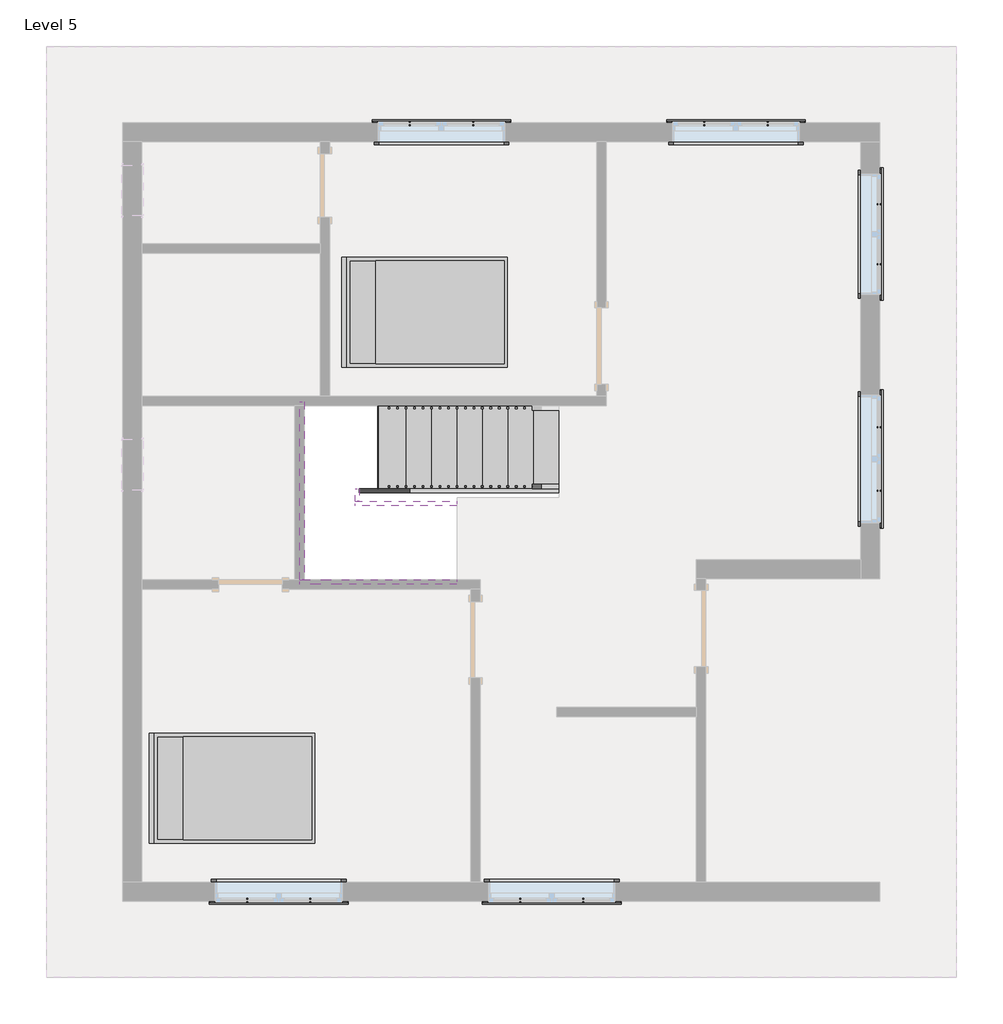
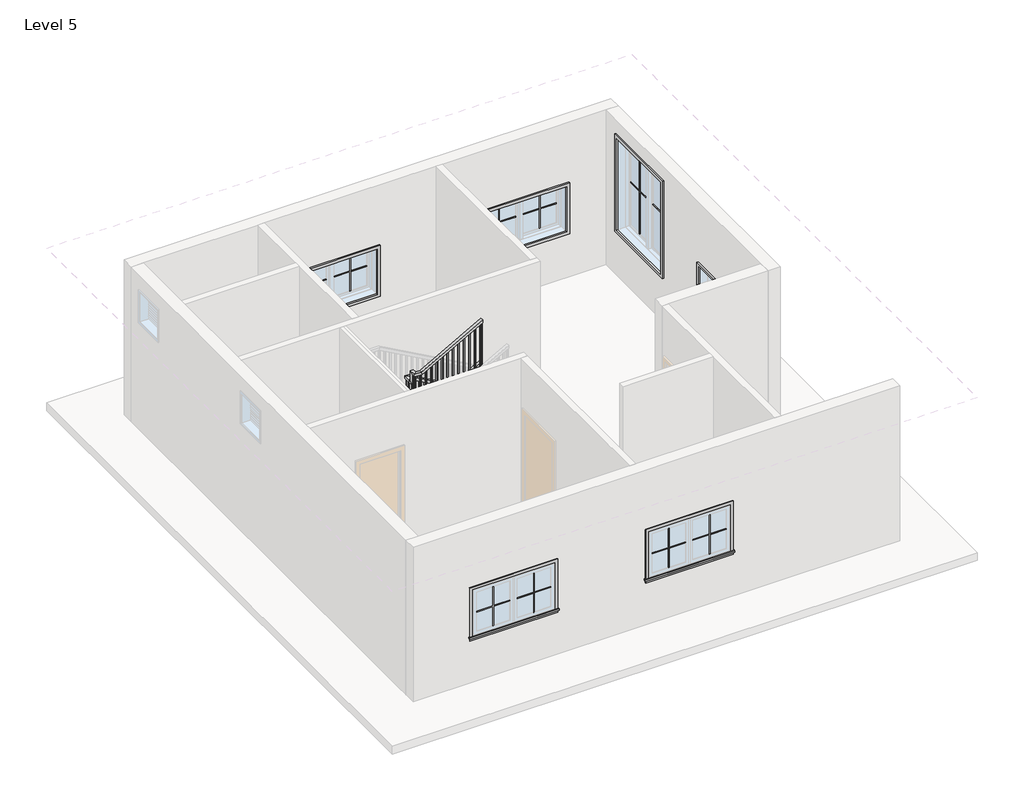
# One storey, part 2 of 2: 24 proxies, 6 members, 2 furniture elements, 1 railing, 1 stair flight.
"""IFC4 building model written with IfcOpenShell, lengths in millimetres."""

from ifc_helpers import new_model, si_unit, frame, origin, place, context, project, spatial, polyline, outline, extrude, faceted_brep, transform, mapped, element, save
from components import muntin_pattern_2x2_muntin_pattern_2x2_9352d081, muntin_pattern_2x2_muntin_pattern_2x2_5c2cbe28, muntin_pattern_2x2_muntin_pattern_2x2_bff912c5, muntin_pattern_2x2_muntin_pattern_2x2_c2194282, trim_window_exterior_flat_with_sill_979bde60, trim_window_exterior_flat_with_sill_e04b3088, trim_window_interior_flat_picture_frame_7883d11b, trim_window_interior_flat_picture_frame_2a7685fe, bed_17739_bed_17739_15c61121, stair_flight_2d4ab5d3

model = new_model("IFC4")

# Units and contexts
model_context = context("Model", 3, world=origin())
ifc_project = project(units=[si_unit("LENGTHUNIT", "METRE", prefix="MILLI")], contexts=[model_context])

# Site, building, storey
site = spatial("IfcSite", under=ifc_project)
building = spatial("IfcBuilding", under=site)
storey = spatial("IfcBuildingStorey", under=building, Name="Level 5", Elevation=12649.2)

# Proxies
placement = place(None, origin())
muntin_pattern_2x2_muntin_pattern_2x2_shape = muntin_pattern_2x2_muntin_pattern_2x2_9352d081(model_context)
element("IfcBuildingElementProxy", 1, Name="Muntin Pattern_2x2 : Muntin Pattern_2x2", ObjectType="Muntin Pattern_2x2 : Muntin Pattern_2x2", at=placement, inside=storey, context=model_context, shape_type="MappedRepresentation", body=[
    mapped(muntin_pattern_2x2_muntin_pattern_2x2_shape, transform((-3542.9505704, -5264.0292021, 13633.45), x_axis=(-1.0, 0.0, 0.0), y_axis=(0.0, -1.0, 0.0), z_axis=(0.0, 0.0, 1.0))),
])
element("IfcBuildingElementProxy", 2, Name="Muntin Pattern_2x2 : Muntin Pattern_2x2", ObjectType="Muntin Pattern_2x2 : Muntin Pattern_2x2", at=placement, inside=storey, context=model_context, shape_type="MappedRepresentation", body=[
    mapped(muntin_pattern_2x2_muntin_pattern_2x2_shape, transform((-272.7005704, -5264.0292021, 13633.45), x_axis=(-1.0, 0.0, 0.0), y_axis=(0.0, -1.0, 0.0), z_axis=(0.0, 0.0, 1.0))),
])
element("IfcBuildingElementProxy", 3, Name="Muntin Pattern_2x2 : Muntin Pattern_2x2", ObjectType="Muntin Pattern_2x2 : Muntin Pattern_2x2", at=placement, inside=storey, context=model_context, shape_type="MappedRepresentation", body=[
    mapped(muntin_pattern_2x2_muntin_pattern_2x2_shape, transform((3269.0119296, 401.7582979, 13633.45), x_axis=(0.0, -1.0, 0.0), y_axis=(1.0, 0.0, 0.0), z_axis=(0.0, 0.0, 1.0))),
])
element("IfcBuildingElementProxy", 4, Name="Muntin Pattern_2x2 : Muntin Pattern_2x2", ObjectType="Muntin Pattern_2x2 : Muntin Pattern_2x2", at=placement, inside=storey, context=model_context, shape_type="MappedRepresentation", body=[
    mapped(muntin_pattern_2x2_muntin_pattern_2x2_shape, transform((1175.0994296, 4038.7207979, 13633.45), x_axis=(1.0, 0.0, 0.0), y_axis=(0.0, 1.0, 0.0), z_axis=(0.0, 0.0, 1.0))),
])
element("IfcBuildingElementProxy", 5, Name="Muntin Pattern_2x2 : Muntin Pattern_2x2", ObjectType="Muntin Pattern_2x2 : Muntin Pattern_2x2", at=placement, inside=storey, context=model_context, shape_type="MappedRepresentation", body=[
    mapped(muntin_pattern_2x2_muntin_pattern_2x2_shape, transform((-2352.3255704, 4038.7207979, 13633.45), x_axis=(1.0, 0.0, 0.0), y_axis=(0.0, 1.0, 0.0), z_axis=(0.0, 0.0, 1.0))),
])
muntin_pattern_2x2_muntin_pattern_2x2_2_shape = muntin_pattern_2x2_muntin_pattern_2x2_5c2cbe28(model_context)
element("IfcBuildingElementProxy", 6, Name="Muntin Pattern_2x2 : Muntin Pattern_2x2", ObjectType="Muntin Pattern_2x2 : Muntin Pattern_2x2", at=placement, inside=storey, context=model_context, shape_type="MappedRepresentation", body=[
    mapped(muntin_pattern_2x2_muntin_pattern_2x2_2_shape, transform((-4301.7755704, -5264.0292021, 13633.45), x_axis=(1.0, 0.0, 0.0), y_axis=(0.0, 1.0, 0.0), z_axis=(0.0, 0.0, 1.0))),
])
element("IfcBuildingElementProxy", 7, Name="Muntin Pattern_2x2 : Muntin Pattern_2x2", ObjectType="Muntin Pattern_2x2 : Muntin Pattern_2x2", at=placement, inside=storey, context=model_context, shape_type="MappedRepresentation", body=[
    mapped(muntin_pattern_2x2_muntin_pattern_2x2_2_shape, transform((-1031.5255704, -5264.0292021, 13633.45), x_axis=(1.0, 0.0, 0.0), y_axis=(0.0, 1.0, 0.0), z_axis=(0.0, 0.0, 1.0))),
])
element("IfcBuildingElementProxy", 8, Name="Muntin Pattern_2x2 : Muntin Pattern_2x2", ObjectType="Muntin Pattern_2x2 : Muntin Pattern_2x2", at=placement, inside=storey, context=model_context, shape_type="MappedRepresentation", body=[
    mapped(muntin_pattern_2x2_muntin_pattern_2x2_2_shape, transform((3269.0119296, -357.0667021, 13633.45), x_axis=(0.0, 1.0, 0.0), y_axis=(-1.0, 0.0, 0.0), z_axis=(0.0, 0.0, 1.0))),
])
element("IfcBuildingElementProxy", 9, Name="Muntin Pattern_2x2 : Muntin Pattern_2x2", ObjectType="Muntin Pattern_2x2 : Muntin Pattern_2x2", at=placement, inside=storey, context=model_context, shape_type="MappedRepresentation", body=[
    mapped(muntin_pattern_2x2_muntin_pattern_2x2_2_shape, transform((1933.9244296, 4038.7207979, 13633.45), x_axis=(-1.0, 0.0, 0.0), y_axis=(0.0, -1.0, 0.0), z_axis=(0.0, 0.0, 1.0))),
])
element("IfcBuildingElementProxy", 10, Name="Muntin Pattern_2x2 : Muntin Pattern_2x2", ObjectType="Muntin Pattern_2x2 : Muntin Pattern_2x2", at=placement, inside=storey, context=model_context, shape_type="MappedRepresentation", body=[
    mapped(muntin_pattern_2x2_muntin_pattern_2x2_2_shape, transform((-1593.5005704, 4038.7207979, 13633.45), x_axis=(-1.0, 0.0, 0.0), y_axis=(0.0, -1.0, 0.0), z_axis=(0.0, 0.0, 1.0))),
])
muntin_pattern_2x2_muntin_pattern_2x2_3_shape = muntin_pattern_2x2_muntin_pattern_2x2_bff912c5(model_context)
element("IfcBuildingElementProxy", 11, Name="Muntin Pattern_2x2 : Muntin Pattern_2x2", ObjectType="Muntin Pattern_2x2 : Muntin Pattern_2x2", at=placement, inside=storey, context=model_context, shape_type="MappedRepresentation", body=[
    mapped(muntin_pattern_2x2_muntin_pattern_2x2_3_shape, transform((3269.0119296, 3075.1082979, 13633.45), x_axis=(0.0, -1.0, 0.0), y_axis=(1.0, 0.0, 0.0), z_axis=(0.0, 0.0, 1.0))),
])
muntin_pattern_2x2_muntin_pattern_2x2_4_shape = muntin_pattern_2x2_muntin_pattern_2x2_c2194282(model_context)
element("IfcBuildingElementProxy", 12, Name="Muntin Pattern_2x2 : Muntin Pattern_2x2", ObjectType="Muntin Pattern_2x2 : Muntin Pattern_2x2", at=placement, inside=storey, context=model_context, shape_type="MappedRepresentation", body=[
    mapped(muntin_pattern_2x2_muntin_pattern_2x2_4_shape, transform((3269.0119296, 2354.3832979, 13633.45), x_axis=(0.0, 1.0, 0.0), y_axis=(-1.0, 0.0, 0.0), z_axis=(0.0, 0.0, 1.0))),
])
trim_window_exterior_flat_with_sill_shape = trim_window_exterior_flat_with_sill_979bde60(model_context)
element("IfcBuildingElementProxy", 13, Name="Trim-Window-Exterior-Flat : with Sill", ObjectType="Trim-Window-Exterior-Flat : with Sill", at=placement, inside=storey, context=model_context, shape_type="MappedRepresentation", body=[
    mapped(trim_window_exterior_flat_with_sill_shape, transform((-3922.3630704, -5273.5542021, 14478.0), x_axis=(1.0, 0.0, 0.0), y_axis=(0.0, 0.0, 1.0), z_axis=(0.0, -1.0, 0.0))),
])
element("IfcBuildingElementProxy", 14, Name="Trim-Window-Exterior-Flat : with Sill", ObjectType="Trim-Window-Exterior-Flat : with Sill", at=placement, inside=storey, context=model_context, shape_type="MappedRepresentation", body=[
    mapped(trim_window_exterior_flat_with_sill_shape, transform((-652.1130704, -5273.5542021, 14478.0), x_axis=(1.0, 0.0, 0.0), y_axis=(0.0, 0.0, 1.0), z_axis=(0.0, -1.0, 0.0))),
])
element("IfcBuildingElementProxy", 15, Name="Trim-Window-Exterior-Flat : with Sill", ObjectType="Trim-Window-Exterior-Flat : with Sill", at=placement, inside=storey, context=model_context, shape_type="MappedRepresentation", body=[
    mapped(trim_window_exterior_flat_with_sill_shape, transform((3278.5369296, 22.3457979, 14478.0), x_axis=(0.0, 1.0, 0.0), y_axis=(0.0, 0.0, 1.0), z_axis=(1.0, 0.0, 0.0))),
])
element("IfcBuildingElementProxy", 16, Name="Trim-Window-Exterior-Flat : with Sill", ObjectType="Trim-Window-Exterior-Flat : with Sill", at=placement, inside=storey, context=model_context, shape_type="MappedRepresentation", body=[
    mapped(trim_window_exterior_flat_with_sill_shape, transform((1554.5119296, 4048.2457979, 14478.0), x_axis=(-1.0, 0.0, 0.0), y_axis=(0.0, 0.0, 1.0), z_axis=(0.0, 1.0, 0.0))),
])
element("IfcBuildingElementProxy", 17, Name="Trim-Window-Exterior-Flat : with Sill", ObjectType="Trim-Window-Exterior-Flat : with Sill", at=placement, inside=storey, context=model_context, shape_type="MappedRepresentation", body=[
    mapped(trim_window_exterior_flat_with_sill_shape, transform((-1972.9130704, 4048.2457979, 14478.0), x_axis=(-1.0, 0.0, 0.0), y_axis=(0.0, 0.0, 1.0), z_axis=(0.0, 1.0, 0.0))),
])
trim_window_exterior_flat_with_sill_2_shape = trim_window_exterior_flat_with_sill_e04b3088(model_context)
element("IfcBuildingElementProxy", 18, Name="Trim-Window-Exterior-Flat : with Sill", ObjectType="Trim-Window-Exterior-Flat : with Sill", at=placement, inside=storey, context=model_context, shape_type="MappedRepresentation", body=[
    mapped(trim_window_exterior_flat_with_sill_2_shape, transform((3278.5369296, 2714.7457979, 15392.4), x_axis=(0.0, 1.0, 0.0), y_axis=(0.0, 0.0, 1.0), z_axis=(1.0, 0.0, 0.0))),
])
trim_window_interior_flat_picture_frame_shape = trim_window_interior_flat_picture_frame_7883d11b(model_context)
element("IfcBuildingElementProxy", 19, Name="Trim-Window-Interior-Flat : Picture Frame", ObjectType="Trim-Window-Interior-Flat : Picture Frame", at=placement, inside=storey, context=model_context, shape_type="MappedRepresentation", body=[
    mapped(trim_window_interior_flat_picture_frame_shape, transform((-3922.3630704, -5044.9542021, 14478.0), x_axis=(-1.0, 0.0, 0.0), y_axis=(0.0, 0.0, 1.0), z_axis=(0.0, 1.0, 0.0))),
])
element("IfcBuildingElementProxy", 20, Name="Trim-Window-Interior-Flat : Picture Frame", ObjectType="Trim-Window-Interior-Flat : Picture Frame", at=placement, inside=storey, context=model_context, shape_type="MappedRepresentation", body=[
    mapped(trim_window_interior_flat_picture_frame_shape, transform((-652.1130704, -5044.9542021, 14478.0), x_axis=(-1.0, 0.0, 0.0), y_axis=(0.0, 0.0, 1.0), z_axis=(0.0, 1.0, 0.0))),
])
element("IfcBuildingElementProxy", 21, Name="Trim-Window-Interior-Flat : Picture Frame", ObjectType="Trim-Window-Interior-Flat : Picture Frame", at=placement, inside=storey, context=model_context, shape_type="MappedRepresentation", body=[
    mapped(trim_window_interior_flat_picture_frame_shape, transform((3049.9369296, 22.3457979, 14478.0), x_axis=(0.0, -1.0, 0.0), y_axis=(0.0, 0.0, 1.0), z_axis=(-1.0, 0.0, 0.0))),
])
element("IfcBuildingElementProxy", 22, Name="Trim-Window-Interior-Flat : Picture Frame", ObjectType="Trim-Window-Interior-Flat : Picture Frame", at=placement, inside=storey, context=model_context, shape_type="MappedRepresentation", body=[
    mapped(trim_window_interior_flat_picture_frame_shape, transform((1554.5119296, 3819.6457979, 14478.0), x_axis=(1.0, 0.0, 0.0), y_axis=(0.0, 0.0, 1.0), z_axis=(0.0, -1.0, 0.0))),
])
element("IfcBuildingElementProxy", 23, Name="Trim-Window-Interior-Flat : Picture Frame", ObjectType="Trim-Window-Interior-Flat : Picture Frame", at=placement, inside=storey, context=model_context, shape_type="MappedRepresentation", body=[
    mapped(trim_window_interior_flat_picture_frame_shape, transform((-1972.9130704, 3819.6457979, 14478.0), x_axis=(1.0, 0.0, 0.0), y_axis=(0.0, 0.0, 1.0), z_axis=(0.0, -1.0, 0.0))),
])
trim_window_interior_flat_picture_frame_2_shape = trim_window_interior_flat_picture_frame_2a7685fe(model_context)
element("IfcBuildingElementProxy", 24, Name="Trim-Window-Interior-Flat : Picture Frame", ObjectType="Trim-Window-Interior-Flat : Picture Frame", at=placement, inside=storey, context=model_context, shape_type="MappedRepresentation", body=[
    mapped(trim_window_interior_flat_picture_frame_2_shape, transform((3049.9369296, 2714.7457979, 15392.4), x_axis=(0.0, -1.0, 0.0), y_axis=(0.0, 0.0, 1.0), z_axis=(-1.0, 0.0, 0.0))),
])

# Furniture
bed_17739_bed_17739_shape = bed_17739_bed_17739_15c61121(model_context)
element("IfcFurniture", 25, ObjectType="Bed_17739 : Bed_17739", at=placement, inside=storey, context=model_context, shape_type="MappedRepresentation", body=[
    mapped(bed_17739_bed_17739_shape, transform((-4455.7630704, -3920.5467683, 12649.2), x_axis=(0.0, 1.0, 0.0), y_axis=(-1.0, 0.0, 0.0), z_axis=(0.0, 0.0, 1.0))),
])
element("IfcFurniture", 26, ObjectType="Bed_17739 : Bed_17739", at=placement, inside=storey, context=model_context, shape_type="MappedRepresentation", body=[
    mapped(bed_17739_bed_17739_shape, transform((-2150.7130704, 1781.2957979, 12649.2), x_axis=(0.0, 1.0, 0.0), y_axis=(-1.0, 0.0, 0.0), z_axis=(0.0, 0.0, 1.0))),
])

# Members
element("IfcMember", 27, ObjectType="Stringer - 2\" Width", at=placement, inside=storey, context=model_context, shape_type="SweptSolid", body=[
    extrude(outline(polyline([(12649.2, -569.5630704), (12856.7983948, -569.5630704), (14183.2428392, -2957.1630704), (13834.5641651, -2957.1630704), (12649.2, -823.5075732), (12649.2, -569.5630704)])), frame((0.0, -384.0542021, 0.0), z_axis=(0.0, 1.0, 0.0), x_axis=(0.0, 0.0, 1.0)), (0.0, 0.0, 1.0), 50.8),
])
element("IfcMember", 28, ObjectType="Stringer - 2\" Width", at=placement, inside=storey, context=model_context, shape_type="SweptSolid", body=[
    extrude(outline(polyline([(-3007.9630704, -333.2542021), (-2957.1630704, -333.2542021), (-2957.1630704, -485.6542021), (-3007.9630704, -485.6542021), (-3007.9630704, -333.2542021)])), frame((0.0, 0.0, 13944.6), z_axis=(0.0, 0.0, 1.0), x_axis=(1.0, 0.0, 0.0)), (0.0, 0.0, 1.0), 304.8),
])
element("IfcMember", 29, ObjectType="Stringer - 2\" Width", at=placement, inside=storey, context=model_context, shape_type="SweptSolid", body=[
    extrude(outline(polyline([(14380.7983948, -3007.9630704), (14032.1197207, -3007.9630704), (14709.453054, -1788.7630704), (15058.1317281, -1788.7630704), (14380.7983948, -3007.9630704)])), frame((0.0, -536.4542021, 0.0), z_axis=(0.0, 1.0, 0.0), x_axis=(0.0, 0.0, 1.0)), (0.0, 0.0, 1.0), 50.8),
])
element("IfcMember", 30, ObjectType="Stringer - 2\" Width", at=placement, inside=storey, context=model_context, shape_type="SweptSolid", body=[
    extrude(outline(polyline([(12649.2, -569.5630704), (12856.7983948, -569.5630704), (14249.4, -3076.2459598), (14249.4, -3617.5630704), (14201.453054, -3617.5630704), (12649.2, -823.5075732), (12649.2, -569.5630704)])), frame((0.0, 657.3457979, 0.0), z_axis=(0.0, 1.0, 0.0), x_axis=(0.0, 0.0, 1.0)), (0.0, 0.0, 1.0), 50.8),
])
element("IfcMember", 31, ObjectType="Stringer - 2\" Width", at=placement, inside=storey, context=model_context, shape_type="SweptSolid", body=[
    extrude(outline(polyline([(-3668.3630704, 708.1457979), (-3617.5630704, 708.1457979), (-3617.5630704, -1425.4542021), (-3668.3630704, -1425.4542021), (-3668.3630704, 708.1457979)])), frame((0.0, 0.0, 13944.6), z_axis=(0.0, 0.0, 1.0), x_axis=(1.0, 0.0, 0.0)), (0.0, 0.0, 1.0), 304.8),
])
element("IfcMember", 32, ObjectType="Stringer - 2\" Width", at=placement, inside=storey, context=model_context, shape_type="SweptSolid", body=[
    extrude(outline(polyline([(14013.9095059, -3668.3630704), (13944.6, -3668.3630704), (13944.6, -3165.4985677), (14709.453054, -1788.7630704), (15058.1317281, -1788.7630704), (14013.9095059, -3668.3630704)])), frame((0.0, -1476.2542021, 0.0), z_axis=(0.0, 1.0, 0.0), x_axis=(0.0, 0.0, 1.0)), (0.0, 0.0, 1.0), 50.8),
])

# Railing
element("IfcRailing", 33, ObjectType="Handrail - Rectangular", at=placement, inside=storey, context=model_context, shape_type="SolidModel", body=[
    faceted_brep([(-569.5630704, -333.2542021, 13732.9333333), (-569.5630704, -333.2542021, 13674.820221), (-569.5630704, -282.4542021, 13674.820221), (-569.5630704, -282.4542021, 13732.9333333), (-2931.7630704, -333.2542021, 15045.2666667), (-2982.5630704, -333.2542021, 15015.3757765), (-2982.5630704, -282.4542021, 15015.3757765), (-2931.7630704, -282.4542021, 15045.2666667), (-2931.7630704, -333.2542021, 15087.6), (-2982.5630704, -333.2542021, 15036.8), (-2982.5630704, -282.4542021, 15036.8), (-2931.7630704, -282.4542021, 15087.6), (-3007.9630704, -333.2542021, 15087.6), (-3007.9630704, -333.2542021, 15036.8), (-3058.7630704, -282.4542021, 15036.8), (-3058.7630704, -282.4542021, 15087.6), (-3007.9630704, -409.4542021, 15087.6), (-3007.9630704, -409.4542021, 15036.8), (-3058.7630704, -409.4542021, 15036.8), (-3058.7630704, -409.4542021, 15087.6), (-3007.9630704, -460.2542021, 15087.6), (-3007.9630704, -511.0542021, 15036.8), (-3058.7630704, -511.0542021, 15036.8), (-3058.7630704, -460.2542021, 15087.6), (-3007.9630704, -460.2542021, 15299.2666667), (-3007.9630704, -511.0542021, 15248.4666667), (-3058.7630704, -511.0542021, 15248.4666667), (-3058.7630704, -460.2542021, 15299.2666667), (-3007.9630704, -536.4542021, 15299.2666667), (-3007.9630704, -536.4542021, 15248.4666667), (-3058.7630704, -587.2542021, 15248.4666667), (-3058.7630704, -587.2542021, 15299.2666667), (-2931.7630704, -536.4542021, 15299.2666667), (-2918.5994682, -536.4542021, 15248.4666667), (-2918.5994682, -587.2542021, 15248.4666667), (-2931.7630704, -587.2542021, 15299.2666667), (-1788.7630704, -536.4542021, 15934.2666667), (-1788.7630704, -587.2542021, 15934.2666667), (-1788.7630704, -587.2542021, 15876.1535543), (-1788.7630704, -536.4542021, 15876.1535543)], [[[0, 1, 2, 3]], [[1, 0, 4, 5]], [[2, 1, 5, 6]], [[3, 2, 6, 7]], [[0, 3, 7, 4]], [[5, 4, 8, 9]], [[6, 5, 9, 10]], [[7, 6, 10, 11]], [[4, 7, 11, 8]], [[9, 8, 12, 13]], [[10, 9, 13, 14]], [[11, 10, 14, 15]], [[8, 11, 15, 12]], [[13, 12, 16, 17]], [[14, 13, 17, 18]], [[15, 14, 18, 19]], [[12, 15, 19, 16]], [[17, 16, 20, 21]], [[18, 17, 21, 22]], [[19, 18, 22, 23]], [[16, 19, 23, 20]], [[21, 20, 24, 25]], [[22, 21, 25, 26]], [[23, 22, 26, 27]], [[20, 23, 27, 24]], [[25, 24, 28, 29]], [[26, 25, 29, 30]], [[27, 26, 30, 31]], [[24, 27, 31, 28]], [[29, 28, 32, 33]], [[30, 29, 33, 34]], [[31, 30, 34, 35]], [[28, 31, 35, 32]], [[36, 37, 38, 39]], [[33, 32, 36, 39]], [[34, 33, 39, 38]], [[35, 34, 38, 37]], [[32, 35, 37, 36]]]),
    extrude(outline(polyline([(15856.7507765, -1823.6880704), (14850.5333333, -1823.6880704), (14850.5333333, -1804.6380704), (15867.3341099, -1804.6380704), (15856.7507765, -1823.6880704)])), frame((0.0, -571.3792021, 0.0), z_axis=(0.0, 1.0, 0.0), x_axis=(0.0, 0.0, 1.0)), (0.0, 0.0, 1.0), 19.05),
    extrude(outline(polyline([(15800.3063321, -1925.2880704), (14850.5333333, -1925.2880704), (14850.5333333, -1906.2380704), (15810.8896654, -1906.2380704), (15800.3063321, -1925.2880704)])), frame((0.0, -571.3792021, 0.0), z_axis=(0.0, 1.0, 0.0), x_axis=(0.0, 0.0, 1.0)), (0.0, 0.0, 1.0), 19.05),
    extrude(outline(polyline([(15743.8618876, -2026.8880704), (14850.5333333, -2026.8880704), (14850.5333333, -2007.8380704), (15754.445221, -2007.8380704), (15743.8618876, -2026.8880704)])), frame((0.0, -571.3792021, 0.0), z_axis=(0.0, 1.0, 0.0), x_axis=(0.0, 0.0, 1.0)), (0.0, 0.0, 1.0), 19.05),
    extrude(outline(polyline([(15687.4174432, -2128.4880704), (14681.2, -2128.4880704), (14681.2, -2109.4380704), (15698.0007765, -2109.4380704), (15687.4174432, -2128.4880704)])), frame((0.0, -571.3792021, 0.0), z_axis=(0.0, 1.0, 0.0), x_axis=(0.0, 0.0, 1.0)), (0.0, 0.0, 1.0), 19.05),
    extrude(outline(polyline([(15630.9729988, -2230.0880704), (14681.2, -2230.0880704), (14681.2, -2211.0380704), (15641.5563321, -2211.0380704), (15630.9729988, -2230.0880704)])), frame((0.0, -571.3792021, 0.0), z_axis=(0.0, 1.0, 0.0), x_axis=(0.0, 0.0, 1.0)), (0.0, 0.0, 1.0), 19.05),
    extrude(outline(polyline([(15574.5285543, -2331.6880704), (14681.2, -2331.6880704), (14681.2, -2312.6380704), (15585.1118876, -2312.6380704), (15574.5285543, -2331.6880704)])), frame((0.0, -571.3792021, 0.0), z_axis=(0.0, 1.0, 0.0), x_axis=(0.0, 0.0, 1.0)), (0.0, 0.0, 1.0), 19.05),
    extrude(outline(polyline([(15518.0841099, -2433.2880704), (14511.8666667, -2433.2880704), (14511.8666667, -2414.2380704), (15528.6674432, -2414.2380704), (15518.0841099, -2433.2880704)])), frame((0.0, -571.3792021, 0.0), z_axis=(0.0, 1.0, 0.0), x_axis=(0.0, 0.0, 1.0)), (0.0, 0.0, 1.0), 19.05),
    extrude(outline(polyline([(15461.6396654, -2534.8880704), (14511.8666667, -2534.8880704), (14511.8666667, -2515.8380704), (15472.2229988, -2515.8380704), (15461.6396654, -2534.8880704)])), frame((0.0, -571.3792021, 0.0), z_axis=(0.0, 1.0, 0.0), x_axis=(0.0, 0.0, 1.0)), (0.0, 0.0, 1.0), 19.05),
    extrude(outline(polyline([(15405.195221, -2636.4880704), (14511.8666667, -2636.4880704), (14511.8666667, -2617.4380704), (15415.7785543, -2617.4380704), (15405.195221, -2636.4880704)])), frame((0.0, -571.3792021, 0.0), z_axis=(0.0, 1.0, 0.0), x_axis=(0.0, 0.0, 1.0)), (0.0, 0.0, 1.0), 19.05),
    extrude(outline(polyline([(15348.7507765, -2738.0880704), (14342.5333333, -2738.0880704), (14342.5333333, -2719.0380704), (15359.3341099, -2719.0380704), (15348.7507765, -2738.0880704)])), frame((0.0, -571.3792021, 0.0), z_axis=(0.0, 1.0, 0.0), x_axis=(0.0, 0.0, 1.0)), (0.0, 0.0, 1.0), 19.05),
    extrude(outline(polyline([(15292.3063321, -2839.6880704), (14342.5333333, -2839.6880704), (14342.5333333, -2820.6380704), (15302.8896654, -2820.6380704), (15292.3063321, -2839.6880704)])), frame((0.0, -571.3792021, 0.0), z_axis=(0.0, 1.0, 0.0), x_axis=(0.0, 0.0, 1.0)), (0.0, 0.0, 1.0), 19.05),
    extrude(outline(polyline([(15235.8618876, -2941.2880704), (14342.5333333, -2941.2880704), (14342.5333333, -2922.2380704), (15246.445221, -2922.2380704), (15235.8618876, -2941.2880704)])), frame((0.0, -571.3792021, 0.0), z_axis=(0.0, 1.0, 0.0), x_axis=(0.0, 0.0, 1.0)), (0.0, 0.0, 1.0), 19.05),
    extrude(outline(polyline([(-3023.8380704, -501.5292021), (-3023.8380704, -520.5792021), (-3042.8880704, -520.5792021), (-3042.8880704, -501.5292021), (-3023.8380704, -501.5292021)])), frame((0.0, 0.0, 14173.2), z_axis=(0.0, 0.0, 1.0), x_axis=(1.0, 0.0, 0.0)), (0.0, 0.0, 1.0), 1075.2666667),
    extrude(outline(polyline([(-3023.8380704, -399.9292021), (-3023.8380704, -418.9792021), (-3042.8880704, -418.9792021), (-3042.8880704, -399.9292021), (-3023.8380704, -399.9292021)])), frame((0.0, 0.0, 14173.2), z_axis=(0.0, 0.0, 1.0), x_axis=(1.0, 0.0, 0.0)), (0.0, 0.0, 1.0), 863.6),
    extrude(outline(polyline([(-2998.4380704, -317.3792021), (-3017.4880704, -317.3792021), (-3017.4880704, -298.3292021), (-2998.4380704, -298.3292021), (-2998.4380704, -317.3792021)])), frame((0.0, 0.0, 14173.2), z_axis=(0.0, 0.0, 1.0), x_axis=(1.0, 0.0, 0.0)), (0.0, 0.0, 1.0), 863.6),
    extrude(outline(polyline([(14978.3341099, -2915.8880704), (14003.8666667, -2915.8880704), (14003.8666667, -2896.8380704), (14967.7507765, -2896.8380704), (14978.3341099, -2915.8880704)])), frame((0.0, -317.3792021, 0.0), z_axis=(0.0, 1.0, 0.0), x_axis=(0.0, 0.0, 1.0)), (0.0, 0.0, 1.0), 19.05),
    extrude(outline(polyline([(14921.8896654, -2814.2880704), (14003.8666667, -2814.2880704), (14003.8666667, -2795.2380704), (14911.3063321, -2795.2380704), (14921.8896654, -2814.2880704)])), frame((0.0, -317.3792021, 0.0), z_axis=(0.0, 1.0, 0.0), x_axis=(0.0, 0.0, 1.0)), (0.0, 0.0, 1.0), 19.05),
    extrude(outline(polyline([(14865.445221, -2712.6880704), (14003.8666667, -2712.6880704), (14003.8666667, -2693.6380704), (14854.8618876, -2693.6380704), (14865.445221, -2712.6880704)])), frame((0.0, -317.3792021, 0.0), z_axis=(0.0, 1.0, 0.0), x_axis=(0.0, 0.0, 1.0)), (0.0, 0.0, 1.0), 19.05),
    extrude(outline(polyline([(14809.0007765, -2611.0880704), (13834.5333333, -2611.0880704), (13834.5333333, -2592.0380704), (14798.4174432, -2592.0380704), (14809.0007765, -2611.0880704)])), frame((0.0, -317.3792021, 0.0), z_axis=(0.0, 1.0, 0.0), x_axis=(0.0, 0.0, 1.0)), (0.0, 0.0, 1.0), 19.05),
    extrude(outline(polyline([(14752.5563321, -2509.4880704), (13834.5333333, -2509.4880704), (13834.5333333, -2490.4380704), (14741.9729988, -2490.4380704), (14752.5563321, -2509.4880704)])), frame((0.0, -317.3792021, 0.0), z_axis=(0.0, 1.0, 0.0), x_axis=(0.0, 0.0, 1.0)), (0.0, 0.0, 1.0), 19.05),
    extrude(outline(polyline([(14696.1118876, -2407.8880704), (13834.5333333, -2407.8880704), (13834.5333333, -2388.8380704), (14685.5285543, -2388.8380704), (14696.1118876, -2407.8880704)])), frame((0.0, -317.3792021, 0.0), z_axis=(0.0, 1.0, 0.0), x_axis=(0.0, 0.0, 1.0)), (0.0, 0.0, 1.0), 19.05),
    extrude(outline(polyline([(14639.6674432, -2306.2880704), (13665.2, -2306.2880704), (13665.2, -2287.2380704), (14629.0841099, -2287.2380704), (14639.6674432, -2306.2880704)])), frame((0.0, -317.3792021, 0.0), z_axis=(0.0, 1.0, 0.0), x_axis=(0.0, 0.0, 1.0)), (0.0, 0.0, 1.0), 19.05),
    extrude(outline(polyline([(14583.2229988, -2204.6880704), (13665.2, -2204.6880704), (13665.2, -2185.6380704), (14572.6396654, -2185.6380704), (14583.2229988, -2204.6880704)])), frame((0.0, -317.3792021, 0.0), z_axis=(0.0, 1.0, 0.0), x_axis=(0.0, 0.0, 1.0)), (0.0, 0.0, 1.0), 19.05),
    extrude(outline(polyline([(14526.7785543, -2103.0880704), (13665.2, -2103.0880704), (13665.2, -2084.0380704), (14516.195221, -2084.0380704), (14526.7785543, -2103.0880704)])), frame((0.0, -317.3792021, 0.0), z_axis=(0.0, 1.0, 0.0), x_axis=(0.0, 0.0, 1.0)), (0.0, 0.0, 1.0), 19.05),
    extrude(outline(polyline([(14470.3341099, -2001.4880704), (13495.8666667, -2001.4880704), (13495.8666667, -1982.4380704), (14459.7507765, -1982.4380704), (14470.3341099, -2001.4880704)])), frame((0.0, -317.3792021, 0.0), z_axis=(0.0, 1.0, 0.0), x_axis=(0.0, 0.0, 1.0)), (0.0, 0.0, 1.0), 19.05),
    extrude(outline(polyline([(14413.8896654, -1899.8880704), (13495.8666667, -1899.8880704), (13495.8666667, -1880.8380704), (14403.3063321, -1880.8380704), (14413.8896654, -1899.8880704)])), frame((0.0, -317.3792021, 0.0), z_axis=(0.0, 1.0, 0.0), x_axis=(0.0, 0.0, 1.0)), (0.0, 0.0, 1.0), 19.05),
    extrude(outline(polyline([(14357.445221, -1798.2880704), (13495.8666667, -1798.2880704), (13495.8666667, -1779.2380704), (14346.8618876, -1779.2380704), (14357.445221, -1798.2880704)])), frame((0.0, -317.3792021, 0.0), z_axis=(0.0, 1.0, 0.0), x_axis=(0.0, 0.0, 1.0)), (0.0, 0.0, 1.0), 19.05),
    extrude(outline(polyline([(14301.0007765, -1696.6880704), (13326.5333333, -1696.6880704), (13326.5333333, -1677.6380704), (14290.4174432, -1677.6380704), (14301.0007765, -1696.6880704)])), frame((0.0, -317.3792021, 0.0), z_axis=(0.0, 1.0, 0.0), x_axis=(0.0, 0.0, 1.0)), (0.0, 0.0, 1.0), 19.05),
    extrude(outline(polyline([(14244.5563321, -1595.0880704), (13326.5333333, -1595.0880704), (13326.5333333, -1576.0380704), (14233.9729988, -1576.0380704), (14244.5563321, -1595.0880704)])), frame((0.0, -317.3792021, 0.0), z_axis=(0.0, 1.0, 0.0), x_axis=(0.0, 0.0, 1.0)), (0.0, 0.0, 1.0), 19.05),
    extrude(outline(polyline([(14188.1118876, -1493.4880704), (13326.5333333, -1493.4880704), (13326.5333333, -1474.4380704), (14177.5285543, -1474.4380704), (14188.1118876, -1493.4880704)])), frame((0.0, -317.3792021, 0.0), z_axis=(0.0, 1.0, 0.0), x_axis=(0.0, 0.0, 1.0)), (0.0, 0.0, 1.0), 19.05),
    extrude(outline(polyline([(14131.6674432, -1391.8880704), (13157.2, -1391.8880704), (13157.2, -1372.8380704), (14121.0841099, -1372.8380704), (14131.6674432, -1391.8880704)])), frame((0.0, -317.3792021, 0.0), z_axis=(0.0, 1.0, 0.0), x_axis=(0.0, 0.0, 1.0)), (0.0, 0.0, 1.0), 19.05),
    extrude(outline(polyline([(14075.2229988, -1290.2880704), (13157.2, -1290.2880704), (13157.2, -1271.2380704), (14064.6396654, -1271.2380704), (14075.2229988, -1290.2880704)])), frame((0.0, -317.3792021, 0.0), z_axis=(0.0, 1.0, 0.0), x_axis=(0.0, 0.0, 1.0)), (0.0, 0.0, 1.0), 19.05),
    extrude(outline(polyline([(14018.7785543, -1188.6880704), (13157.2, -1188.6880704), (13157.2, -1169.6380704), (14008.195221, -1169.6380704), (14018.7785543, -1188.6880704)])), frame((0.0, -317.3792021, 0.0), z_axis=(0.0, 1.0, 0.0), x_axis=(0.0, 0.0, 1.0)), (0.0, 0.0, 1.0), 19.05),
    extrude(outline(polyline([(13962.3341099, -1087.0880704), (12987.8666667, -1087.0880704), (12987.8666667, -1068.0380704), (13951.7507765, -1068.0380704), (13962.3341099, -1087.0880704)])), frame((0.0, -317.3792021, 0.0), z_axis=(0.0, 1.0, 0.0), x_axis=(0.0, 0.0, 1.0)), (0.0, 0.0, 1.0), 19.05),
    extrude(outline(polyline([(13905.8896654, -985.4880704), (12987.8666667, -985.4880704), (12987.8666667, -966.4380704), (13895.3063321, -966.4380704), (13905.8896654, -985.4880704)])), frame((0.0, -317.3792021, 0.0), z_axis=(0.0, 1.0, 0.0), x_axis=(0.0, 0.0, 1.0)), (0.0, 0.0, 1.0), 19.05),
    extrude(outline(polyline([(13849.445221, -883.8880704), (12987.8666667, -883.8880704), (12987.8666667, -864.8380704), (13838.8618876, -864.8380704), (13849.445221, -883.8880704)])), frame((0.0, -317.3792021, 0.0), z_axis=(0.0, 1.0, 0.0), x_axis=(0.0, 0.0, 1.0)), (0.0, 0.0, 1.0), 19.05),
    extrude(outline(polyline([(13793.0007765, -782.2880704), (12818.5333333, -782.2880704), (12818.5333333, -763.2380704), (13782.4174432, -763.2380704), (13793.0007765, -782.2880704)])), frame((0.0, -317.3792021, 0.0), z_axis=(0.0, 1.0, 0.0), x_axis=(0.0, 0.0, 1.0)), (0.0, 0.0, 1.0), 19.05),
    extrude(outline(polyline([(13736.5563321, -680.6880704), (12818.5333333, -680.6880704), (12818.5333333, -661.6380704), (13725.9729988, -661.6380704), (13736.5563321, -680.6880704)])), frame((0.0, -317.3792021, 0.0), z_axis=(0.0, 1.0, 0.0), x_axis=(0.0, 0.0, 1.0)), (0.0, 0.0, 1.0), 19.05),
    extrude(outline(polyline([(-3023.8380704, -552.3292021), (-3023.8380704, -571.3792021), (-3042.8880704, -571.3792021), (-3042.8880704, -552.3292021), (-3023.8380704, -552.3292021)])), frame((0.0, 0.0, 14173.2), z_axis=(0.0, 0.0, 1.0), x_axis=(1.0, 0.0, 0.0)), (0.0, 0.0, 1.0), 1075.2666667),
    extrude(outline(polyline([(-3023.8380704, -317.3792021), (-3042.8880704, -317.3792021), (-3042.8880704, -298.3292021), (-3023.8380704, -298.3292021), (-3023.8380704, -317.3792021)])), frame((0.0, 0.0, 14173.2), z_axis=(0.0, 0.0, 1.0), x_axis=(1.0, 0.0, 0.0)), (0.0, 0.0, 1.0), 863.6),
    extrude(outline(polyline([(15865.570221, -1807.8130704), (14850.5333333, -1807.8130704), (14850.5333333, -1788.7630704), (15876.1535543, -1788.7630704), (15865.570221, -1807.8130704)])), frame((0.0, -571.3792021, 0.0), z_axis=(0.0, 1.0, 0.0), x_axis=(0.0, 0.0, 1.0)), (0.0, 0.0, 1.0), 19.05),
    extrude(outline(polyline([(13685.4035543, -588.6130704), (12818.5333333, -588.6130704), (12818.5333333, -569.5630704), (13674.820221, -569.5630704), (13685.4035543, -588.6130704)])), frame((0.0, -317.3792021, 0.0), z_axis=(0.0, 1.0, 0.0), x_axis=(0.0, 0.0, 1.0)), (0.0, 0.0, 1.0), 19.05),
])

# Stair flight
stair_flight_shape = stair_flight_2d4ab5d3(model_context)
element("IfcStairFlight", 34, ObjectType="2\" Tread 1\" Nosing 1/4\" Riser", at=placement, inside=storey, context=model_context, shape_type="MappedRepresentation", body=[
    mapped(stair_flight_shape, transform((0.0, 0.0, 0.0), x_axis=(1.0, 0.0, 0.0), y_axis=(0.0, 1.0, 0.0), z_axis=(0.0, 0.0, 1.0))),
])

save(model, "model.ifc")

# Revit data of these elements
# Type "Muntin Pattern_2x2 : Muntin Pattern_2x2"
#   Width [instance default] = 4' - 0"
#   Thickness = 0' - 0 1/2"
#   Height [instance default] = 4' - 0"
#   Distance = 0' - 0 3/4"
#   Interior Material [instance default] = none
#   Exterior Material [instance default] = none
#   Default Elevation = 0
# Type "Trim-Window-Exterior-Flat : with Sill"
#   Trim Width = 0' - 2 1/4"
#   Trim Thickness_Picture Frame = 0' - 1 1/4"
#   Trim Thickness_with Sill = 0' - 0 3/4"
#   Sill Thickness = 0' - 1 1/4"
#   Opening Width [instance default] = 2' - 0"
#   Opening Height [instance default] = 3' - 0"
#   Default Elevation = 4' - 0"
#   Sill = yes
#   Picture Frame = no
#   Trim Material [instance default] = none
# Type "Trim-Window-Interior-Flat : Picture Frame"
#   Trim Thickness_Picture Frame = 0' - 1 1/4"
#   Trim Width = 0' - 2 1/4"
#   Trim Thickness_with Sill = 0' - 0 3/4"
#   Sill Thickness = 0' - 1 1/4"
#   Opening Width [instance default] = 2' - 0"
#   Opening Height [instance default] = 3' - 0"
#   Default Elevation = 4' - 0"
#   Sill = no
#   Picture Frame = yes
#   Trim Material [instance default] = none
# Type "Bed_17739 : Bed_17739"
#   Default Elevation = 0
# Type "Handrail - Rectangular"
#   Assembly Code = "C2010400"
#   built-in parameter 1008612 = 0.0416667 (stored number, unit not read)
#   built-in parameter 1008611 = 0.0416667 (stored number, unit not read)
#   built-in parameter 1008609 = 0.333333 (stored number, unit not read)
#   built-in parameter 1008604 = 0.166667 (stored number, unit not read)
#   built-in parameter 1008603 = 0.166667 (stored number, unit not read)
#   Railing Height = 3' - 0"
#   built-in parameter 1008630 = 2
#   built-in parameter 1008610 = 2
#   built-in parameter 1008618 = Baluster - Square : 3/4"
# Elements 1, 2, 3, 4, 5, 6, 7, 8, 9, 10 (IfcBuildingElementProxy, "Muntin Pattern_2x2 : Muntin Pattern_2x2")
#   Width = 2' - 0 5/8"
#   Height = 2' - 6 1/2"
#   Interior Material = Wood - Stained
#   Exterior Material = Clad - White
#   Phase Created = New Construction
#   Materials on its faces: "Clad - White", "Wood - Stained"
# Elements 11, 12 (IfcBuildingElementProxy, "Muntin Pattern_2x2 : Muntin Pattern_2x2")
#   Width = 1' - 11 1/8"
#   Height = 5' - 6 1/2"
#   Interior Material = Wood - Stained
#   Exterior Material = Clad - White
#   Phase Created = New Construction
#   Materials on its faces: "Clad - White", "Wood - Stained"
# Elements 13, 14, 15, 16, 17 (IfcBuildingElementProxy, "Trim-Window-Exterior-Flat : with Sill")
#   Opening Width = 5' - 0"
#   Opening Height = 3' - 0"
#   Trim Material = Clad - White
#   Phase Created = New Construction
#   Materials on its faces: "Clad - White"
# Element 18 (IfcBuildingElementProxy, "Trim-Window-Exterior-Flat : with Sill")
#   Opening Width = 4' - 9"
#   Opening Height = 6' - 0"
#   Trim Material = Clad - White
#   Phase Created = New Construction
#   Materials on its faces: "Clad - White"
# Elements 19, 20, 21, 22, 23 (IfcBuildingElementProxy, "Trim-Window-Interior-Flat : Picture Frame")
#   Opening Width = 5' - 0"
#   Opening Height = 3' - 0"
#   Trim Material = Wood - Stained
#   Phase Created = New Construction
#   Materials on its faces: "Wood - Stained"
# Element 24 (IfcBuildingElementProxy, "Trim-Window-Interior-Flat : Picture Frame")
#   Opening Width = 4' - 9"
#   Opening Height = 6' - 0"
#   Trim Material = Wood - Stained
#   Phase Created = New Construction
#   Materials on its faces: "Wood - Stained"
# Elements 25, 26 (IfcFurniture, "Bed_17739 : Bed_17739")
#   Phase Created = New Construction
#   Materials on its faces: "legs", "sheets", "bed frame", "Blanket"
# Elements 27, 28, 29, 30, 31, 32 (IfcMember, "Stringer - 2\" Width")
#   Phase Created = New Construction
# Element 33 (IfcRailing, "Handrail - Rectangular")
#   Phase Created = New Construction
# Element 34 (IfcStairFlight, "2\" Tread 1\" Nosing 1/4\" Riser")
#   Phase Created = New Construction
# Materials
#   "Clad - White": class "Wood", colour RGB 242 242 238, transparency 0, Cost = 0
#   "Wood - Stained": class "Wood", colour RGB 224 178 126, transparency 0, Cost = 0
#   "legs": colour RGB 90 73 37, transparency 0, Cost = 0
#   "sheets": colour RGB 200 195 176, transparency 0, Cost = 0
#   "bed frame": colour RGB 90 73 37, transparency 0, Cost = 0
#   "Blanket": class "System", colour RGB 59 0 1, transparency 0, Cost = 0
